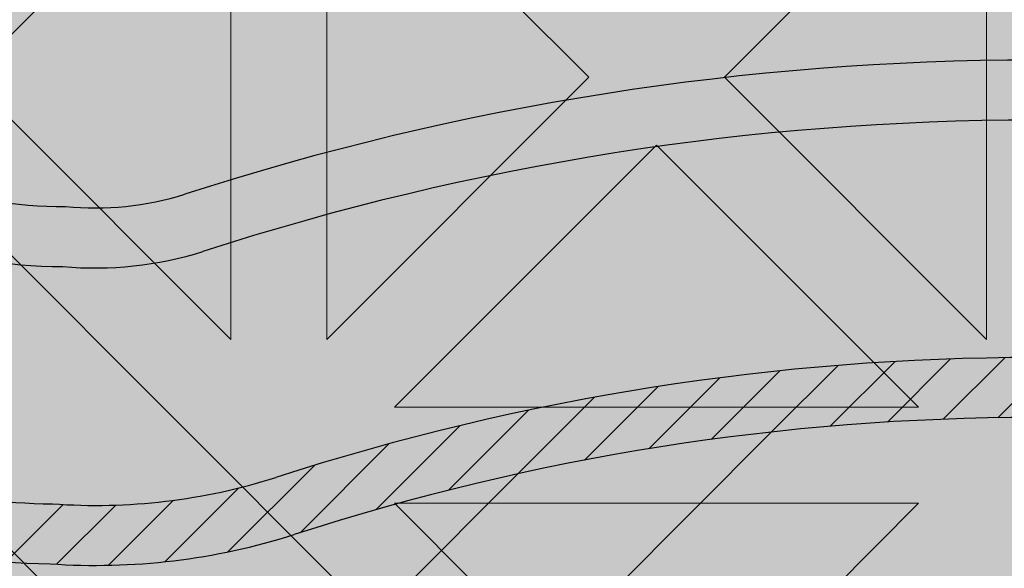
# Model space of a CAD drawing. Units: inches. Extents: x 844 to 2234, y 346 to 1084.
# Tile 20 of 93: x 1120.159 to 1122.777, y 703.603 to 705.06. Entities that reach past the tile are written whole.
import ezdxf

# ---------------------------------------------------------------- set-up
doc = ezdxf.new("R2010")
doc.units = ezdxf.units.IN
doc.header["$MEASUREMENT"] = 0
for name, color, linetype, lineweight in [('A-ANNO-DIMS', 2, 'Continuous', 18), ('furniture', 8, 'Continuous', 18), ('RA-AP-01$0$INT', 35, 'Continuous', 5)]:
    doc.layers.add(name, color=color, linetype=linetype, lineweight=lineweight)
doc.layers.add('RA-AP-01$0$FURN', color=3, linetype='Continuous')
doc.layers.add('RA-AP-01$0$WOOD', color=64, linetype='Continuous')
doc.styles.get("Standard").update_dxf_attribs({"font": 'arial.ttf'})
doc.dimstyles.get("Standard").update_dxf_attribs({"dimtxt": 6, "dimasz": 3, "dimexe": 0.18, "dimexo": 0.0625, "dimgap": 0.09, "dimtad": 0, "dimtih": 1, "dimtoh": 1, "dimdec": 1, "dimzin": 0, "dimdsep": 46, "dimlunit": 3, "dimtxsty": 'Standard', "dimblk": 'ARCHTICK', "dimcen": 0.09, "dimadec": 0, "dimazin": 0, "dimtfac": 1, "dimtdec": 1, "dimtofl": 0, "dimtmove": 0, "dimatfit": 3, "dimfxl": 1, "dimtolj": 1, "dimtzin": 0, "dimarcsym": 0})

# ---------------------------------------------------------------- blocks, each defined once
blk = doc.blocks.new('A$C18D01794')
at = {"layer": 'RA-AP-01$0$INT'}
h = blk.add_hatch(color=256, dxfattribs=at)
h.paths.add_polyline_path([(4.585917135068448, -7.856712009587804), (4.614201406330596, -7.856712009587056), (4.668846067270487, -7.802067348644738), (4.723490728212344, -7.856712009584164), (4.771774999457151, -7.856712009582887), (4.826419660396886, -7.80206734864072), (4.862780050090322, -7.838427738332541), (4.844495778842715, -7.856712009580965), (4.862780050090411, -7.856712009580482), (4.905206456960182, -7.814285602707865), (4.947632863832445, -7.856712009578238), (4.965917135079675, -7.856712009577755), (4.947632863831759, -7.838427738330656), (4.983993253523576, -7.802067348637219), (5.038637914464627, -7.856712009575829), (5.08692218571208, -7.856712009574554), (5.141566846649976, -7.802067348634224), (5.196211507589851, -7.856712009571666), (5.224495778822615, -7.856712009570916), (4.905206456953975, -7.537422687702283)])
h.paths.add_polyline_path([(4.895206456956031, -7.575706958950402), (4.895206456958921, -7.684996280828174), (4.840561796018589, -7.630351619890275)], flags=16)
h.paths.add_polyline_path([(4.915206456955638, -7.575706958949956), (4.969851117895509, -7.630351619887399), (4.915206456957609, -7.684996280827732)], flags=16)
h.paths.add_polyline_path([(4.826419660395175, -7.644493755514321), (4.881064321335613, -7.699138416452331), (4.771774999456703, -7.69913841645522)], flags=16)
h.paths.add_polyline_path([(4.983993253519558, -7.644493755510815), (5.038637914460456, -7.699138416449285), (4.929348592581548, -7.69913841645126)], flags=16)
h.paths.add_polyline_path([(4.881064321336025, -7.719138416452334), (4.826419660397532, -7.773783077393256), (4.771774999457062, -7.719138416455217)], flags=16)
h.paths.add_polyline_path([(4.929348592582019, -7.71913841645126), (5.038637914460982, -7.719138416449284), (4.983993253522945, -7.773783077389749)], flags=16)
h.paths.add_polyline_path([(4.895206456960191, -7.733280552075633), (4.895206456962115, -7.806001331460164), (4.876922185715016, -7.824285602708492), (4.840561796021581, -7.787925213016675)], flags=16)
h.paths.add_polyline_path([(4.915206456958487, -7.733280552075187), (4.969851117899527, -7.787925213013798), (4.933490728206909, -7.824285602708034), (4.9152064569598, -7.806001331461736)], flags=16)
h.paths.add_polyline_path([(4.757632863832376, -7.733280552079264), (4.812277524772842, -7.787925213017304), (4.757632863834348, -7.842569873958233)], flags=16)
h.paths.add_polyline_path([(4.737632863832376, -7.73328055207979), (4.737632863834348, -7.842569873958701), (4.682988202893906, -7.787925213020692)], flags=16)
h.paths.add_polyline_path([(5.05278005008503, -7.733280552072701), (5.052780050087917, -7.842569873951664), (4.998135389146995, -7.787925213013169)], flags=16)
h.paths.add_polyline_path([(5.072780050085024, -7.733280552072333), (5.127424711025931, -7.787925213010806), (5.072780050087916, -7.842569873951244)], flags=16)
h.paths.add_polyline_path([(4.935917135072783, -7.506712009583784), (5.255206456948811, -7.826001331459767), (5.255206456948932, -7.797717060211899), (5.200561796010279, -7.743072399273238), (5.255206456949403, -7.688427738334128), (5.25520645694961, -7.640143467086677), (5.200561796009787, -7.585498806146837), (5.236922185702417, -7.549138416454212), (5.255206456949919, -7.56742268770172), (5.255206456949998, -7.549138416454178), (5.212780050078687, -7.506712009583814), (5.25520645695036, -7.464285602712145), (5.255206456950438, -7.446001331464763), (5.236922185702424, -7.464285602712779), (5.200561796009796, -7.427925213020149), (5.255206456950753, -7.373280552079203), (5.25520645695096, -7.324996280834394), (5.200561796010322, -7.270351619893748), (5.255206456951428, -7.215706958952649), (5.255206456951547, -7.187422687705071)])
h.paths.add_polyline_path([(5.042988202883395, -7.42792521302065), (5.097632863823085, -7.373280552080975), (5.097632863822622, -7.482569873959883)], flags=16)
h.paths.add_polyline_path([(5.028846067259663, -7.442067348644384), (5.083490728198774, -7.496712009583504), (4.974201406321001, -7.496712009583035)], flags=16)
h.paths.add_polyline_path([(5.117632863823087, -7.37328055208089), (5.172277524762331, -7.42792521302015), (5.11763286382262, -7.482569873959851)], flags=16)
h.paths.add_polyline_path([(5.08349072819877, -7.516712009582191), (5.028846067259652, -7.571356670521302), (4.974201406320998, -7.516712009582638)], flags=16)
h.paths.add_polyline_path([(5.131774999446817, -7.35913841645716), (5.186419660386065, -7.413783077396415), (5.241064321325782, -7.359138416456712)], flags=17)
h.paths.add_polyline_path([(5.131774999446228, -7.496712009583703), (5.186419660386065, -7.442067348643883), (5.222780050079488, -7.478427738337313), (5.204495778832781, -7.496712009584014)], flags=16)
h.paths.add_polyline_path([(5.097632863822613, -7.530854145205813), (5.097632863823061, -7.640143467084723), (5.042988202883383, -7.585498806145032)], flags=16)
h.paths.add_polyline_path([(5.131774999446899, -7.339138416457162), (5.241064321325809, -7.339138416456712), (5.186419660386591, -7.284493755517479)], flags=17)
h.paths.add_polyline_path([(5.131774999446226, -7.516712009581999), (5.204495778830767, -7.516712009581702), (5.22278005007868, -7.534996280829206), (5.186419660386049, -7.571356670521828)], flags=16)
h.paths.add_polyline_path([(5.11763286382262, -7.530854145205852), (5.17227752476232, -7.585498806145562), (5.117632863823064, -7.64014346708481)], flags=16)
h.paths.add_polyline_path([(5.186419660386069, -7.599640941770585), (5.241064321325754, -7.654285602710281), (5.131774999446791, -7.654285602709814)], flags=16)
h.paths.add_polyline_path([(5.131774999446872, -7.674285602709813), (5.24106432132578, -7.674285602710282), (5.186419660386554, -7.728930263649504)], flags=16)
h.paths.add_polyline_path([(5.255206456951811, -7.126001331467467), (5.255206456951895, -7.106712009588038), (4.555206456956052, -7.106712009588038), (4.555206456956136, -7.12600133146746), (4.905206456953973, -7.476001331465289)])
h.paths.add_polyline_path([(4.983993253513404, -7.368930263651977), (4.92934859257295, -7.314285602713969), (5.03863791445186, -7.314285602711063)], flags=16)
h.paths.add_polyline_path([(4.969851117889988, -7.383072399276016), (4.915206456952556, -7.437717060215906), (4.915206456949648, -7.328427738338133)], flags=16)
h.paths.add_polyline_path([(4.929348592572535, -7.294285602713971), (4.983993253511019, -7.239640941773039), (5.038637914451496, -7.294285602711065)], flags=16)
h.paths.add_polyline_path([(5.052780050074912, -7.280143467087016), (4.998135389134438, -7.225498806148989), (5.052780050072919, -7.170854145208052)], flags=16)
h.paths.add_polyline_path([(5.07278005007491, -7.280143467086489), (5.072780050072918, -7.170854145207579), (5.127424711013374, -7.225498806145578)], flags=16)
h.paths.add_polyline_path([(4.89520645695295, -7.437717060216355), (4.840561796013067, -7.383072399278919), (4.895206456950961, -7.328427738338582)], flags=16)
h.paths.add_polyline_path([(4.915206456948365, -7.280143467090674), (4.915206456946434, -7.207422687704125), (4.933490728192729, -7.18913841645701), (4.969851117886972, -7.225498806149623)], flags=16)
h.paths.add_polyline_path([(4.881064321327021, -7.314285602715054), (4.82641966038902, -7.368930263655506), (4.771774999448108, -7.314285602717047)], flags=16)
h.paths.add_polyline_path([(4.895206456950073, -7.280143467091125), (4.840561796009022, -7.225498806152518), (4.876922185700835, -7.18913841645908), (4.895206456948749, -7.207422687706589)], flags=16)
h.paths.add_polyline_path([(4.983993253510392, -7.211356670525576), (4.947632863816944, -7.174996280833758), (4.965917135064043, -7.156712009585847), (5.038637914448995, -7.156712009584522)], flags=16)
h.paths.add_polyline_path([(4.881064321326543, -7.294285602715056), (4.771774999447578, -7.294285602717046), (4.826419660385607, -7.239640941776569)], flags=16)
h.paths.add_polyline_path([(4.905206456946447, -7.19913841645844), (4.862780050074785, -7.156712009587725), (4.947632863816685, -7.156712009586302)], flags=16)
h.paths.add_polyline_path([(5.14156684663679, -7.211356670521528), (5.086922185696452, -7.156712009583639), (5.196211507574223, -7.156712009581651)], flags=16)
h.paths.add_polyline_path([(4.8264196603837, -7.211356670529104), (4.771774999442643, -7.156712009590501), (4.8444957788276, -7.156712009588568), (4.862780050075511, -7.17499628083566)], flags=16)
h.paths.add_polyline_path([(4.812277524760289, -7.225498806153156), (4.757632863822258, -7.28014346709363), (4.757632863819352, -7.170854145214669)], flags=16)
h.paths.add_polyline_path([(4.73763286382226, -7.280143467093997), (4.682988202881349, -7.22549880615554), (4.737632863819352, -7.170854145215086)], flags=16)
h.paths.add_polyline_path([(4.723490728195188, -7.156712009591787), (4.668846067257299, -7.211356670532127), (4.614201406317417, -7.156712009594693)], flags=16)
h.paths.add_polyline_path([(4.597632863829262, -7.506712009583814), (4.555206456957951, -7.54913841645418), (4.555206456958029, -7.56742268770172), (4.573490728205535, -7.549138416454212), (4.609851117898167, -7.585498806146839), (4.555206456958338, -7.640143467086675), (4.555206456958546, -7.688427738334125), (4.60985111789767, -7.743072399273238), (4.555206456959015, -7.797717060211899), (4.555206456959138, -7.826001331459767), (4.874495778835167, -7.506712009583786), (4.5552064569564, -7.187422687705062), (4.555206456956523, -7.215706958952644), (4.609851117897629, -7.270351619893746), (4.555206456956988, -7.324996280834396), (4.555206456957198, -7.373280552079195), (4.609851117898153, -7.427925213020147), (4.573490728205528, -7.464285602712779), (4.555206456957507, -7.446001331464756), (4.555206456957585, -7.464285602712143)])
h.paths.add_polyline_path([(4.712780050085332, -7.482569873959882), (4.712780050084863, -7.373280552080972), (4.767424711024555, -7.42792521302065)], flags=16)
h.paths.add_polyline_path([(4.726922185709173, -7.496712009583504), (4.781566846648288, -7.442067348644384), (4.836211507586949, -7.496712009583033)], flags=16)
h.paths.add_polyline_path([(4.692780050085327, -7.482569873959851), (4.638135389145619, -7.427925213020149), (4.692780050084865, -7.373280552080892)], flags=16)
h.paths.add_polyline_path([(4.726922185709182, -7.516712009582191), (4.836211507586949, -7.51671200958264), (4.7815668466483, -7.571356670521304)], flags=16)
h.paths.add_polyline_path([(4.678637914461726, -7.496712009583706), (4.605917135075169, -7.496712009584014), (4.587632863828464, -7.478427738337311), (4.623993253521887, -7.442067348643881)], flags=16)
h.paths.add_polyline_path([(4.712780050085336, -7.530854145205816), (4.767424711024568, -7.585498806145034), (4.71278005008489, -7.640143467084724)], flags=16)
h.paths.add_polyline_path([(4.678637914461726, -7.516712009582001), (4.623993253521899, -7.571356670521829), (4.587632863829271, -7.534996280829206), (4.605917135077185, -7.5167120095817)], flags=16)
h.paths.add_polyline_path([(4.692780050085336, -7.530854145205848), (4.692780050084889, -7.64014346708481), (4.638135389145632, -7.585498806145562)], flags=16)
h.paths.add_polyline_path([(4.623993253521885, -7.413783077396415), (4.678637914461131, -7.359138416457161), (4.56934859258217, -7.359138416456712)], flags=17)
h.paths.add_polyline_path([(4.623993253521901, -7.599640941770568), (4.678637914461158, -7.654285602709814), (4.569348592582195, -7.654285602710281)], flags=16)
h.paths.add_polyline_path([(4.678637914461051, -7.339138416457162), (4.623993253521361, -7.284493755517479), (4.569348592582143, -7.339138416456712)], flags=17)
h.paths.add_polyline_path([(4.678637914461076, -7.674285602709813), (4.623993253521399, -7.728930263649504), (4.569348592582167, -7.674285602710281)], flags=16)
h = blk.add_hatch(color=256, dxfattribs=at)
h.paths.add_polyline_path([(4.905206456954232, -7.537422687702028), (4.874495778835232, -7.506712009583718), (4.555206456959138, -7.826001331459766), (4.555206456959269, -7.856712009588616), (4.585917135068449, -7.856712009587804)])
h.paths.add_polyline_path([(4.935917135072152, -7.506712009583152), (4.905206456953497, -7.537422687701806), (5.224495778822614, -7.856712009570917), (5.255206456948681, -7.856712009570104), (5.255206456948813, -7.826001331459768)])
h.paths.add_polyline_path([(5.255206456951549, -7.18742268770507), (5.255206456951813, -7.126001331467461), (4.905206456953563, -7.476001331465701), (4.935917135072559, -7.506712009584006)])
h.paths.add_polyline_path([(4.874495778835167, -7.506712009583785), (4.905206456953818, -7.476001331465132), (4.555206456956135, -7.126001331467458), (4.555206456956399, -7.187422687705064)])
h = blk.add_hatch(color=256, dxfattribs=at)
h.paths.add_polyline_path([(4.969851117891331, -7.630351619889621), (4.915206456952669, -7.575706958950966), (4.915206456952222, -7.684996280828739)])
h.paths.add_polyline_path([(4.895206456953064, -7.575706958950968), (4.840561796014413, -7.630351619889628), (4.895206456953533, -7.684996280828741)])
h.paths.add_polyline_path([(4.826419660390684, -7.644493755513362), (4.771774999451003, -7.699138416453052), (4.881064321329913, -7.699138416452587)])
h.paths.add_polyline_path([(4.881064321329884, -7.719138416452585), (4.771774999450921, -7.719138416453052), (4.82641966039018, -7.773783077392298)])
h.paths.add_polyline_path([(4.895206456953734, -7.733280552076196), (4.840561796013912, -7.787925213016031), (4.876922185707337, -7.824285602709455), (4.895206456954043, -7.806001331462747)])
h.paths.add_polyline_path([(4.862780050082808, -7.838427738332388), (4.826419660390178, -7.802067348639763), (4.771774999450351, -7.856712009579595), (4.844495778835303, -7.856712009579895)])
h.paths.add_polyline_path([(4.812277524766446, -7.787925213016036), (4.757632863827191, -7.733280552076788), (4.757632863826741, -7.842569873955747)])
h.paths.add_polyline_path([(4.737632863827191, -7.733280552076863), (4.682988202887508, -7.787925213016558), (4.737632863826743, -7.842569873955778)])
h.paths.add_polyline_path([(4.668846067263777, -7.802067348640287), (4.614201406325123, -7.856712009578949), (4.723490728202894, -7.856712009579402)])
h.paths.add_polyline_path([(4.905206456953846, -7.814285602708654), (4.862780050082654, -7.856712009579847), (4.947632863824561, -7.85671200958032)])
h.paths.add_polyline_path([(4.915206456952028, -7.733280552076195), (4.91520645695173, -7.806001331460731), (4.933490728199234, -7.824285602708648), (4.96985111789186, -7.787925213016022)])
h.paths.add_polyline_path([(5.038637914454841, -7.719138416453029), (4.929348592575874, -7.71913841645258), (4.983993253515593, -7.773783077392289)])
h.paths.add_polyline_path([(4.983993253515065, -7.644493755513352), (4.929348592575849, -7.699138416452582), (5.038637914454755, -7.699138416453031)])
h.paths.add_polyline_path([(5.052780050079843, -7.73328055207676), (4.998135389140595, -7.787925213016018), (5.052780050080309, -7.842569873955721)])
h.paths.add_polyline_path([(4.983993253516868, -7.802067348639752), (4.947632863824241, -7.838427738332383), (4.965917135071747, -7.856712009579888), (5.038637914456701, -7.856712009579572)])
h.paths.add_polyline_path([(5.127424711019533, -7.787925213016519), (5.072780050079843, -7.733280552076838), (5.07278005008031, -7.842569873955751)])
h.paths.add_polyline_path([(5.141566846643269, -7.802067348640248), (5.086922185704154, -7.85671200957937), (5.196211507581929, -7.856712009578901)])
for p, q in [((4.874495778835167, -7.506712009583786), (4.555206456959136, -7.826001331459769)), ((4.905206456953975, -7.537422687702283), (4.585917135071132, -7.856712009585121)), ((4.826419660395171, -7.644493755514321), (4.771774999456703, -7.69913841645522)), ((4.881064321335613, -7.699138416452333), (4.826419660395173, -7.64449375551432)), ((4.771774999456703, -7.69913841645522), (4.881064321335613, -7.699138416452333)), ((4.771774999457064, -7.719138416455219), (4.881064321336027, -7.719138416452333)), ((4.771774999457064, -7.719138416455219), (4.826419660397532, -7.773783077393256)), ((4.881064321336027, -7.719138416452333), (4.826419660397532, -7.773783077393256)), ((4.682988202893908, -7.78792521302069), (4.737632863832376, -7.733280552079792)), ((4.737632863832376, -7.733280552079792), (4.737632863834348, -7.842569873958701)), ((4.757632863832376, -7.733280552079266), (4.812277524772842, -7.787925213017302)), ((4.757632863832376, -7.733280552079266), (4.757632863834348, -7.842569873958229)), ((4.895206456960191, -7.73328055207563), (4.840561796021581, -7.787925213016675)), ((4.895206456962113, -7.806001331460581), (4.895206456960191, -7.73328055207563)), ((4.737632863834348, -7.842569873958701), (4.682988202893906, -7.787925213020692)), ((4.757632863834348, -7.842569873958229), (4.812277524772842, -7.787925213017302)), ((4.840561796021581, -7.787925213016674), (4.876922185715016, -7.824285602708492))]:
    blk.add_line(p, q, dxfattribs=at)
blk = doc.blocks.new('A$C32926AE1')
at = {"layer": 'RA-AP-01$0$WOOD'}
h = blk.add_hatch(color=256, dxfattribs=at)
h.dxf.hatch_style = 1
h.paths.add_polyline_path([(5.157430609644524, 4.573483066760929, -0.1009492694046607), (5.155401577623758, 4.593365984175333, -0.1842662638101597), (5.172249623284174, 4.638795604568598, 0.2056608120311276), (5.179560981299304, 4.661316324430096, 0.3614336704623542), (5.134352340494423, 4.706524965234944, 0.2056608120311297), (5.111831620632933, 4.699213607219793, -0.1842662638101113), (5.066402000239693, 4.682365561559342, -0.1055311479399994), (5.045656153913092, 4.68467289944697, 0.1567636581983829), (4.763886414745334, 4.684672899446966, -0.1055311479399895), (4.743140568418733, 4.68236556155934, -0.1842662638100833), (4.6977109480255, 4.69921360721979, 0.2056608120302612), (4.675190228164109, 4.706524965234949, 0.3614336704708441), (4.629981587358889, 4.66131632442871, 0.2056608120245944), (4.637292945374126, 4.638795604567974, -0.1842662638101024), (4.654140991034615, 4.59336598417475, -0.1009492694055169), (4.652111959013835, 4.573483066760181, 0.021410119221476), (4.629748025606143, 4.156712009541676, 0.0214101192214795), (4.652111959013809, 3.739940952323101, -0.1009492694059586), (4.654140991034615, 3.720058034908448, -0.1842662638100975), (4.637292945374126, 3.674628414515226, 0.2056608120245705), (4.629981587358889, 3.652107694654492, 0.3614336704708879), (4.675190228164113, 3.606899053848249, 0.2056608120302384), (4.697710948025501, 3.614210411863408, -0.1842662638100995), (4.743140568418738, 3.63105845752386, -0.1055311479402541), (4.763886414745388, 3.628751119636215, 0.1567636581983776), (5.045656153913137, 3.628751119636244, -0.1055311479397538), (5.066402000239692, 3.631058457523857, -0.1842662638101067), (5.111831620632931, 3.614210411863407, 0.2056608120310924), (5.134352340494417, 3.606899053848256, 0.3614336704624001), (5.179560981299307, 3.652107694653103, 0.2056608120311314), (5.172249623284175, 3.6746284145146, -0.1842662638101402), (5.155401577623758, 3.72005803490786, -0.1009492694051366), (5.15743060964455, 3.739940952322354, 0.0214101192215073), (5.179794543052287, 4.156712009541468, 0.0214101192215252)])
h.paths.add_polyline_path([(4.639748609479751, 4.156712009541513, 0.0213537860821624), (4.661970494867118, 3.741887061152232, -0.094075836301374), (4.664143710413708, 3.7196126951003, -0.1824818158568985), (4.644813765429836, 3.668037719127816, 0.2056608120245319), (4.639939526753007, 3.653023905887301, 0.3614336704710246), (4.676106439397173, 3.616856993242342, 0.2056608120302234), (4.691120252638095, 3.621731231919122, -0.1824818158602558), (4.742695228611606, 3.641061176902986, -0.1029891339458722), (4.766991894714349, 3.638256818950944, 0.156709409989566), (5.042550673941472, 3.638256818950105, -0.102989133958497), (5.066847340047078, 3.641061176902949, -0.1824818158594995), (5.118422316020358, 3.621731231919103, 0.2056608120311416), (5.133436129261316, 3.616856993242346, 0.3614336704621468), (5.169603041905217, 3.653023905886178, 0.2056608120310986), (5.164728803228477, 3.668037719127177, -0.1824818158565612), (5.145398858244737, 3.719612695099578, -0.0940758363009313), (5.147572073791232, 3.741887061151398, 0.0213537860822023), (5.169793959178681, 4.156712009541451, 0.0213537860822226), (5.147572073791203, 4.571536957931898, -0.0940758363005034), (5.145398858244737, 4.59381132398362, -0.1824818158565587), (5.164728803228476, 4.645386299956021, 0.2056608120311045), (5.169603041905216, 4.66040011319702, 0.3614336704621845), (5.133436129261313, 4.696567025840856, 0.2056608120310773), (5.118422316020359, 4.691692787164098, -0.182481815859508), (5.066847340047078, 4.67236284218025, -0.1029891339584606), (5.04255067394148, 4.675167200133092, 0.156709409989566), (4.766991894714357, 4.675167200132257, -0.1029891339458842), (4.742695228611611, 4.672362842180213, -0.1824818158602725), (4.691120252638095, 4.691692787164077, 0.2056608120302152), (4.676106439397174, 4.696567025840858, 0.3614336704710363), (4.639939526753005, 4.660400113195899, 0.2056608120245495), (4.644813765429837, 4.645386299955384, -0.1824818158568934), (4.664143710413708, 4.593811323982902, -0.0940758363009187), (4.661970494867149, 4.571536957931074, 0.021353786082177)], flags=16)
h.paths.add_polyline_path([(5.129794543052235, 4.432167055276933, -0.0141661062790638), (5.130152669293814, 4.156927903047693, -0.0141661062790647), (5.129794543052234, 3.881688750818433, -0.0785247771143638), (5.10979738006795, 3.755143611847103, 0.0945969212073497), (5.105408519571111, 3.717898134952927, 0.1043170707844957), (5.116074640131521, 3.670385395016088, 0.1043170707864965), (5.068561900193738, 3.681051515576561, 0.09459692119553), (5.031316423304057, 3.676662655080835, -0.1580239521427272), (4.778226145355827, 3.676662655080367, 0.0945969211986668), (4.740980668464973, 3.681051515576592, 0.1043170707882822), (4.693467928526415, 3.670385395015844, 0.1043170707867916), (4.704134049087309, 3.717898134953662, 0.0945969211972894), (4.69974518859162, 3.755143611844042, -0.0785247771163196), (4.679748025606343, 3.881688750818406, -0.0141661062790663), (4.679389899364763, 4.156927903047693, -0.0141661062790672), (4.679748025606343, 4.432167055276998, -0.0785247771163064), (4.699745188591625, 4.55871219425134, 0.094596921197333), (4.704134049087308, 4.595957671141738, 0.1043170707867205), (4.693467928526416, 4.643470411079523, 0.1043170707882628), (4.740980668464965, 4.632804290518776, 0.0945969211988114), (4.778226145355874, 4.637193151015016, -0.158023952142669), (5.031316423304015, 4.637193151014546, 0.0945969211956361), (5.068561900193736, 4.632804290518806, 0.1043170707864979), (5.11607464013152, 4.643470411079278, 0.1043170707844617), (5.105408519571112, 4.595957671142455, 0.0945969212074597), (5.109797380067959, 4.558712194248236, -0.0785247771143467)], flags=0)
h.paths.add_polyline_path([(5.119794532311105, 4.432259799204851, -0.0142000800617244), (5.120156169157484, 4.156927903047701, -0.0142000800617277), (5.119794532311105, 3.881596006890482, -0.0784894509520253), (5.100273383573699, 3.758192358677797, 0.0940138827242913), (5.095413455884425, 3.717477693979438, 0.0606271852308753), (5.099615656341024, 3.686844378806616, 0.0606271852322524), (5.068982341167493, 3.691046579263239, 0.0940138827010453), (5.028267676478798, 3.686186651576848, -0.1580706864508061), (4.781274892180912, 3.686186651576435, 0.0940138827026903), (4.740560227491556, 3.691046579263279, 0.0606271852339895), (4.709926912317155, 3.686844378806508, 0.0606271852329405), (4.714129112773991, 3.717477693980356, 0.094013882701304), (4.709269185087677, 3.758192358669163, -0.0784894509577193), (4.689748036347473, 3.881596006890469, -0.014200080061729), (4.689386399501094, 4.156927903047709, -0.0142000800617217), (4.689748036347473, 4.432259799204808, -0.078489450957724), (4.709269185087651, 4.555663447426125, 0.0940138827014585), (4.714129112773992, 4.596378112114996, 0.0606271852329731), (4.709926912317154, 4.62701142728886, 0.0606271852340196), (4.74056022749157, 4.622809226832087, 0.0940138827024997), (4.781274892180847, 4.627669154518912, -0.1580706864508359), (5.028267676478777, 4.627669154518526, 0.0940138827010946), (5.068982341167492, 4.622809226832129, 0.060627185232254), (5.099615656341024, 4.627011427288751, 0.0606271852308727), (5.095413455884425, 4.59637811211593, 0.0940138827241088), (5.100273383573675, 4.555663447417647, -0.0784894509520978)], flags=0)
h.paths.add_polyline_path([(5.06978912287499, 4.430218106756144, -0.014241683694547), (5.070173729147532, 4.156927903047672, -0.0142416836945458), (5.06978912287499, 3.883637699339223, -0.0800609523125196), (5.052662118612511, 3.773463122773442, 0.0526421978001116), (5.04590916754064, 3.740550867606997, 0.0526421977992423), (5.012996912374707, 3.73379791653534, -0.1583028414718258), (4.796545656286308, 3.73379791653451, 0.0526421978034211), (4.763633401117837, 3.740550867607021, 0.0526421978018622), (4.756880450045755, 3.773463122774558, -0.0800609523117106), (4.739753445783639, 3.883637699339268, -0.0142416836945435), (4.739368839511098, 4.156927903047671, -0.0142416836945477), (4.739753445783639, 4.430218106756155, -0.0800609523116345), (4.75688045004574, 4.540392683320762, 0.052642197801941), (4.763633401117837, 4.573304938488346, 0.0526421978035071), (4.796545656286361, 4.580057889560873, -0.1583028414717561), (5.012996912374669, 4.580057889560039, 0.0526421977993048), (5.04590916754064, 4.57330493848837, 0.0526421978002057), (5.052662118612529, 4.540392683321868, -0.080060952312477)], flags=0)
h.paths.add_polyline_path([(5.049789715110557, 4.43038092723357, -0.0143097550741839), (5.05018085590259, 4.156927903047715, -0.0143097550741854), (5.049789715110558, 3.883474878861827, -0.0800685599149176), (5.03362098255317, 3.779581877367999, 0.0306258898956367), (5.028241146483733, 3.758218888663947, 0.0306258898977031), (5.006878157778253, 3.75283905259408, -0.1583983521624096), (4.802664410878162, 3.752839052594731, 0.0306258898946014), (4.781301422174808, 3.758218888663924, 0.0306258898967912), (4.775921586105202, 3.779581877368794, -0.080068559914251), (4.759752853548071, 3.883474878861786, -0.0143097550741854), (4.759361712756037, 4.156927903047671, -0.0143097550741854), (4.759752853548071, 4.430380927233557, -0.0800685599142479), (4.775921586105193, 4.534273928726546, 0.0306258898968306), (4.781301422174808, 4.555636917431444, 0.0306258898945754), (4.802664410878143, 4.561016753500631, -0.1583983521624168), (5.006878157778244, 4.561016753501291, 0.0306258898977177), (5.028241146483733, 4.555636917431421, 0.0306258898958182), (5.03362098255321, 4.534273928727244, -0.080068559914796)], flags=0)
h.paths.add_polyline_path([(4.999766070382627, 4.428171244713864, -0.0143443147609634), (5.000198441819402, 4.156927903047689, -0.0143443147609612), (4.999766070382627, 3.885684561381556, -0.0784641635803329), (4.987356730658798, 3.799103304488872, -0.1506053783831347), (4.822185837999821, 3.79910330448882, -0.0784641635803318), (4.809776498276007, 3.885684561381509, -0.014344314760963), (4.809344126839227, 4.156927903047677, -0.0143443147609645), (4.809776498276007, 4.428171244713873, -0.0784641635803192), (4.822185837999822, 4.514752501606549, -0.1506053783831338), (4.987356730658798, 4.514752501606494, -0.078464163580285)], flags=0)
h.paths.add_polyline_path([(4.979755254238824, 4.42764379880488, -0.0143772539198268), (4.980205517789977, 4.156927903047693, -0.0143772539198275), (4.979755254238824, 3.886212007290489, -0.0689242507424422), (4.971183264704897, 3.815276770442801, -0.1296645318904179), (4.838359303953726, 3.815276770442746, -0.0689242507424186), (4.829787314419809, 3.886212007290419, -0.0143772539198292), (4.829337050868653, 4.156927903047653, -0.0143772539198325), (4.829787314419809, 4.427643798804946, -0.0689242507424211), (4.838359303953725, 4.498579035652621, -0.1296645318904187), (4.971183264704897, 4.498579035652565, -0.0689242507424401)], flags=0)
h = blk.add_hatch(color=256, dxfattribs=at)
h.dxf.hatch_style = 1
h.paths.add_polyline_path([(5.145398858244737, 4.59381132398362, -0.1824818158565616), (5.164728803228476, 4.645386299956021, 0.2056608120311045), (5.169603041905216, 4.66040011319702, 0.3614336704621845), (5.133436129261313, 4.696567025840856, 0.2056608120310773), (5.118422316020359, 4.691692787164098, -0.182481815859508), (5.066847340047078, 4.67236284218025, -0.1029891339584606), (5.04255067394148, 4.675167200133092, 0.156709409989566), (4.766991894714357, 4.675167200132257, -0.1029891339458842), (4.742695228611611, 4.672362842180213, -0.1824818158602725), (4.691120252638095, 4.691692787164077, 0.2056608120302152), (4.676106439397174, 4.696567025840858, 0.3614336704710363), (4.639939526753005, 4.660400113195899, 0.2056608120245495), (4.644813765429837, 4.645386299955384, -0.1824818158568934), (4.664143710413708, 4.593811323982902, -0.0940758363009187), (4.661970494867149, 4.571536957931074, 0.0213537860821772), (4.639748609479751, 4.156712009541507, 0.0213537860821625), (4.661970494867119, 3.741887061152226, -0.0940758363013071), (4.664143710413708, 3.719612695100309, -0.1824818158569294), (4.644813765429836, 3.668037719127816, 0.2056608120245319), (4.639939526753007, 3.653023905887301, 0.3614336704710246), (4.676106439397173, 3.616856993242342, 0.2056608120302234), (4.691120252638095, 3.621731231919122, -0.1824818158602558), (4.742695228611606, 3.641061176902986, -0.1029891339458722), (4.766991894714349, 3.638256818950944, 0.156709409989566), (5.042550673941472, 3.638256818950105, -0.102989133958497), (5.066847340047078, 3.641061176902949, -0.1824818158594995), (5.118422316020358, 3.621731231919103, 0.2056608120311416), (5.133436129261316, 3.616856993242346, 0.3614336704621468), (5.169603041905217, 3.653023905886178, 0.2056608120310986), (5.164728803228477, 3.668037719127177, -0.1824818158565612), (5.145398858244737, 3.719612695099578, -0.0940758363009313), (5.147572073791232, 3.741887061151398, 0.0213537860822023), (5.169793959178681, 4.156712009541451, 0.0213537860822226), (5.147572073791203, 4.571536957931898, -0.0940758363004996)])
h.paths.add_polyline_path([(5.109797380067958, 4.55871219424824, -0.0785247771143472), (5.129794543052234, 4.432167055276936, -0.0141661062790644), (5.130152669293814, 4.156927903047685, -0.014166106279066), (5.129794543052234, 3.881688750818401, -0.0785247771143517), (5.109797380067946, 3.755143611847092, 0.0945969212073132), (5.105408519571111, 3.717898134952929, 0.1043170707844995), (5.116074640131521, 3.670385395016088, 0.1043170707864965), (5.068561900193738, 3.681051515576561, 0.09459692119553), (5.031316423304057, 3.676662655080835, -0.1580239521427272), (4.778226145355827, 3.676662655080367, 0.0945969211986668), (4.740980668464973, 3.681051515576592, 0.1043170707882822), (4.693467928526415, 3.670385395015844, 0.1043170707867916), (4.704134049087309, 3.717898134953662, 0.0945969211972894), (4.69974518859162, 3.755143611844042, -0.0785247771163196), (4.679748025606343, 3.881688750818406, -0.0141661062790663), (4.679389899364763, 4.156927903047693, -0.0141661062790672), (4.679748025606343, 4.432167055276998, -0.0785247771163064), (4.699745188591625, 4.55871219425134, 0.094596921197333), (4.704134049087308, 4.595957671141738, 0.1043170707867205), (4.693467928526416, 4.643470411079523, 0.1043170707882628), (4.740980668464965, 4.632804290518776, 0.0945969211988114), (4.778226145355874, 4.637193151015016, -0.158023952142669), (5.031316423304015, 4.637193151014546, 0.0945969211956361), (5.068561900193736, 4.632804290518806, 0.1043170707864979), (5.11607464013152, 4.643470411079278, 0.1043170707844617), (5.105408519571112, 4.595957671142455, 0.0945969212074504)], flags=16)
h.paths.add_polyline_path([(5.100273383573655, 4.55566344741771, -0.0784894509521388), (5.119794532311105, 4.432259799204852, -0.0142000800617252), (5.120156169157484, 4.156927903047686, -0.014200080061726), (5.119794532311105, 3.881596006890502, -0.0784894509520446), (5.100273383573696, 3.758192358677786, 0.0940138827242721), (5.095413455884425, 3.717477693979436, 0.0606271852308692), (5.099615656341024, 3.686844378806616, 0.0606271852322522), (5.068982341167493, 3.691046579263239, 0.0940138827010453), (5.028267676478798, 3.686186651576848, -0.1580706864508061), (4.781274892180912, 3.686186651576435, 0.0940138827026903), (4.740560227491556, 3.691046579263279, 0.0606271852339895), (4.709926912317155, 3.686844378806508, 0.0606271852329405), (4.714129112773991, 3.717477693980356, 0.094013882701304), (4.709269185087677, 3.758192358669163, -0.0784894509577193), (4.689748036347473, 3.881596006890469, -0.014200080061729), (4.689386399501094, 4.156927903047709, -0.0142000800617217), (4.689748036347473, 4.432259799204808, -0.078489450957724), (4.709269185087651, 4.555663447426125, 0.0940138827014585), (4.714129112773992, 4.596378112114996, 0.0606271852329731), (4.709926912317154, 4.62701142728886, 0.0606271852340196), (4.74056022749157, 4.622809226832087, 0.0940138827024997), (4.781274892180847, 4.627669154518912, -0.1580706864508359), (5.028267676478777, 4.627669154518526, 0.0940138827010946), (5.068982341167492, 4.622809226832129, 0.060627185232254), (5.099615656341024, 4.627011427288751, 0.0606271852308727), (5.095413455884425, 4.59637811211593, 0.094013882723957)], flags=0)
h.paths.add_polyline_path([(5.04590916754064, 4.57330493848837, 0.0526421978002057), (5.052662118612529, 4.540392683321868, -0.0800609523124783), (5.06978912287499, 4.430218106756142, -0.0142416836945469), (5.070173729147532, 4.156927903047672, -0.0142416836945458), (5.06978912287499, 3.883637699339223, -0.0800609523125196), (5.052662118612511, 3.773463122773442, 0.0526421978001116), (5.04590916754064, 3.740550867606997, 0.0526421977992423), (5.012996912374707, 3.73379791653534, -0.1583028414718258), (4.796545656286308, 3.73379791653451, 0.0526421978034211), (4.763633401117837, 3.740550867607021, 0.0526421978018622), (4.756880450045755, 3.773463122774558, -0.0800609523117106), (4.739753445783639, 3.883637699339268, -0.0142416836945435), (4.739368839511098, 4.156927903047671, -0.0142416836945477), (4.739753445783639, 4.430218106756155, -0.0800609523116345), (4.75688045004574, 4.540392683320762, 0.052642197801941), (4.763633401117837, 4.573304938488346, 0.0526421978035071), (4.796545656286361, 4.580057889560873, -0.1583028414717561), (5.012996912374669, 4.580057889560039, 0.0526421977993048)], flags=0)
h.paths.add_polyline_path([(5.028241146483733, 4.555636917431422, 0.0306258898956949), (5.033620982553182, 4.534273928727329, -0.0800685599148649), (5.049789715110557, 4.430380927233569, -0.0143097550741839), (5.05018085590259, 4.156927903047715, -0.0143097550741854), (5.049789715110558, 3.883474878861827, -0.0800685599149176), (5.03362098255317, 3.779581877367999, 0.0306258898956367), (5.028241146483733, 3.758218888663947, 0.0306258898977031), (5.006878157778253, 3.75283905259408, -0.1583983521624096), (4.802664410878162, 3.752839052594731, 0.0306258898946014), (4.781301422174808, 3.758218888663924, 0.0306258898967912), (4.775921586105202, 3.779581877368794, -0.080068559914251), (4.759752853548071, 3.883474878861786, -0.0143097550741854), (4.759361712756037, 4.156927903047671, -0.0143097550741854), (4.759752853548071, 4.430380927233557, -0.0800685599142479), (4.775921586105193, 4.534273928726546, 0.0306258898968306), (4.781301422174808, 4.555636917431444, 0.0306258898945754), (4.802664410878143, 4.561016753500631, -0.1583983521624168), (5.006878157778244, 4.561016753501291, 0.0306258898977174)], flags=0)
h.paths.add_polyline_path([(4.987356730658798, 4.514752501606494, -0.0784641635803018), (4.999766070382627, 4.428171244713845, -0.0143443147609637), (5.000198441819402, 4.156927903047665, -0.0143443147609622), (4.999766070382628, 3.885684561381514, -0.0784641635802952), (4.987356730658797, 3.799103304488872, -0.1506053783831338), (4.822185837999821, 3.799103304488819, -0.0784641635803342), (4.809776498276007, 3.885684561381512, -0.0143443147609628), (4.809344126839227, 4.156927903047676, -0.0143443147609646), (4.809776498276007, 4.428171244713873, -0.0784641635803192), (4.822185837999822, 4.514752501606549, -0.1506053783831338)], flags=0)
h.paths.add_polyline_path([(4.971183264704897, 4.498579035652566, -0.0689242507424384), (4.979755254238824, 4.427643798804883, -0.0143772539198276), (4.980205517789977, 4.15692790304768, -0.0143772539198258), (4.979755254238823, 3.88621200729051, -0.0689242507424628), (4.971183264704897, 3.815276770442801, -0.129664531890417), (4.838359303953726, 3.815276770442746, -0.0689242507424186), (4.829787314419809, 3.886212007290419, -0.0143772539198292), (4.829337050868653, 4.156927903047653, -0.0143772539198325), (4.829787314419809, 4.427643798804946, -0.0689242507424211), (4.838359303953725, 4.498579035652621, -0.1296645318904187)], flags=0)
h = blk.add_hatch(dxfattribs=at)
h.set_pattern_fill('ANSI31', color=256, scale=0.05, style=0)
h.set_pattern_definition([(45, (0, 0), (-0.0044194173824159, 0.0044194173824159), [])])
h.paths.add_polyline_path([(5.130152669293814, 4.156927903047704, 0.0141661062790657), (5.129794543052234, 4.432167055276982, 0.0777827904001433), (5.110168979996553, 4.557559993161921, -0.0976515123401879), (5.105408519571111, 4.595957671142454, -0.1043170707844687), (5.116074640131522, 4.64347041107928), (5.099615656341024, 4.627011427288751, 0.0606271852308727), (5.095413455884425, 4.59637811211593, 0.0940138827241088), (5.100273383573675, 4.555663447417647, -0.0784894509520972), (5.119794532311105, 4.432259799204852, -0.0142000800617252), (5.120156169157484, 4.156927903047686, -0.014200080061726), (5.119794532311105, 3.881596006890502, -0.0784894509520446), (5.100273383573696, 3.758192358677786, 0.0940138827242721), (5.095413455884425, 3.717477693979436, 0.0606271852308692), (5.099615656341024, 3.686844378806616), (5.116074640131519, 3.67038539501609, -0.1043170707844594), (5.105408519571112, 3.717898134952912, -0.0976515123401594), (5.11016897999655, 3.756295812933435, 0.0777827904001654), (5.129794543052234, 3.881688750818409, 0.0141661062790665)])
h.paths.add_polyline_path([(5.030164222210597, 3.676291055149937, -0.0976515123472002), (5.068561900193739, 3.681051515576561, -0.1043170707864927), (5.116074640131521, 3.670385395016088), (5.099615656341024, 3.686844378806616, 0.0606271852322522), (5.068982341167493, 3.691046579263239, 0.0940138827010453), (5.028267676478798, 3.686186651576848, -0.1580706864508061), (4.781274892180912, 3.686186651576435, 0.0940138827026903), (4.740560227491556, 3.691046579263279, 0.0606271852339913), (4.709926912317154, 3.686844378806508), (4.693467928526416, 3.670385395015845, -0.1043170707882796), (4.740980668464973, 3.681051515576592, -0.0976515123427246), (4.779378346446416, 3.676291055150394, 0.156512506893803)])
h.paths.add_polyline_path([(4.689748036347473, 3.881596006890472, -0.014200080061729), (4.689386399501094, 4.156927903047712, -0.0142000800617195), (4.689748036347473, 4.432259799204768, -0.078489450957742), (4.709269185087648, 4.555663447426114, 0.0940138827014821), (4.714129112773992, 4.596378112114995, 0.0606271852329748), (4.709926912317154, 4.62701142728886), (4.693467928526414, 4.643470411079524, -0.1043170707867939), (4.704134049087309, 4.595957671141706, -0.09765151234893), (4.699373588660725, 4.557559993157876, 0.0777827903975372), (4.679748025606343, 4.432167055276987, 0.0141661062790675), (4.679389899364763, 4.156927903047675, 0.0141661062790641), (4.679748025606343, 3.88168875081843, 0.0777827903975637), (4.699373588660724, 3.756295812937497, -0.0976515123490278), (4.704134049087308, 3.717898134953629, -0.1043170707867196), (4.693467928526416, 3.670385395015845), (4.709926912317155, 3.686844378806508, 0.0606271852329413), (4.714129112773991, 3.717477693980357, 0.0940138827013084), (4.709269185087676, 3.758192358669166, -0.0784894509577192)])
h.paths.add_polyline_path([(4.779378346446434, 4.63756475094498, -0.0976515123427943), (4.740980668464964, 4.632804290518776, -0.1043170707882609), (4.693467928526416, 4.643470411079523), (4.709926912317154, 4.62701142728886, 0.0606271852340196), (4.74056022749157, 4.622809226832087, 0.0940138827024997), (4.781274892180847, 4.627669154518912, -0.1580706864508359), (5.028267676478777, 4.627669154518526, 0.0940138827010946), (5.068982341167492, 4.622809226832129, 0.060627185232254), (5.099615656341024, 4.627011427288751), (5.116074640131521, 4.643470411079279, -0.1043170707865022), (5.068561900193735, 4.632804290518806, -0.0976515123475899), (5.030164222210446, 4.637564750945479, 0.1565125068936924)])
h = blk.add_hatch(dxfattribs=at)
h.set_pattern_fill('ANSI32', color=256, scale=0.2, style=0)
h.set_pattern_definition([(45, (0, 0), (-0.0530330085889911, 0.0530330085889911), []), (45, (0.035355339, 0), (-0.0530330085889911, 0.0530330085889911), [])])
h.paths.add_polyline_path([(5.119794532311105, 4.432259799204823, 0.0777015974868765), (5.10065834347252, 4.554469821747928, -0.0968902511992216), (5.095413455884425, 4.596378112115931, -0.060627185230871), (5.099615656341024, 4.627011427288751, -0.060627185232254), (5.068982341167492, 4.622809226832129, -0.0968902512198245), (5.027074050790956, 4.628054114423209, 0.1564657949319105), (4.782468517866163, 4.628054114422785, -0.0968902512152247), (4.740560227491555, 4.622809226832088, -0.0606271852339878), (4.709926912317155, 4.627011427288859, -0.0606271852329413), (4.714129112773991, 4.596378112115011, -0.0968902512205338), (4.708884225182929, 4.554469821738175, 0.0777015974804443), (4.689748036347473, 4.43225979920482, 0.0142000800617215), (4.689386399501094, 4.156927903047726, 0.0142000800617273), (4.689748036347473, 3.88159600689052, 0.077701597480541), (4.708884225182985, 3.759385984357019, -0.096890251220082), (4.714129112773992, 3.717477693980371, -0.0606271852329731), (4.709926912317154, 3.686844378806507, -0.060627185233988), (4.740560227491554, 3.691046579263279, -0.0968902512152569), (4.782468517866175, 3.685801691672578, 0.1564657949319236), (5.027074050790988, 3.685801691672169, -0.0968902512197451), (5.068982341167491, 3.691046579263239, -0.0606271852322557), (5.099615656341024, 3.686844378806616, -0.0606271852308727), (5.095413455884425, 3.717477693979438, -0.0968902511991229), (5.100658343472507, 3.7593859843474, 0.0777015974868745), (5.119794532311105, 3.8815960068905, 0.014200080061726), (5.120156169157484, 4.156927903047685, 0.0142000800617238)])
h.paths.add_polyline_path([(5.070173729147531, 4.156927903047684, -0.0142416836945481), (5.06978912287499, 3.883637699339191, -0.0800609523125107), (5.052662118612505, 3.773463122773424, 0.0526421978000811), (5.04590916754064, 3.740550867606997, 0.0526421977993214), (5.012996912374658, 3.733797916535325, -0.1583028414717916), (4.796545656286304, 3.733797916534512, 0.0526421978034138), (4.763633401117837, 3.740550867607021, 0.0526421978018622), (4.756880450045755, 3.773463122774558, -0.0800609523117106), (4.739753445783639, 3.883637699339268, -0.0142416836945435), (4.739368839511098, 4.156927903047671, -0.0142416836945477), (4.739753445783639, 4.430218106756155, -0.0800609523116345), (4.75688045004574, 4.540392683320762, 0.052642197801941), (4.763633401117837, 4.573304938488346, 0.0526421978035071), (4.796545656286361, 4.580057889560873, -0.1583028414717561), (5.012996912374669, 4.580057889560039, 0.0526421977993048), (5.04590916754064, 4.57330493848837, 0.0526421978002057), (5.052662118612529, 4.540392683321868, -0.0800609523124783), (5.06978912287499, 4.430218106756142, -0.0142416836945463)], flags=16)
h.paths.add_polyline_path([(5.050180855902591, 4.156927903047686, -0.0143097550741856), (5.049789715110558, 3.883474878861795, -0.0800685599148126), (5.033620982553202, 3.7795818773681, 0.0306258898957837), (5.028241146483733, 3.758218888663947, 0.0306258898977031), (5.006878157778253, 3.75283905259408, -0.1583983521624096), (4.802664410878162, 3.752839052594731, 0.0306258898946014), (4.781301422174808, 3.758218888663924, 0.0306258898967912), (4.775921586105202, 3.779581877368794, -0.080068559914251), (4.759752853548071, 3.883474878861786, -0.0143097550741854), (4.759361712756037, 4.156927903047671, -0.0143097550741854), (4.759752853548071, 4.430380927233557, -0.0800685599142479), (4.775921586105193, 4.534273928726546, 0.0306258898968306), (4.781301422174808, 4.555636917431444, 0.0306258898945754), (4.802664410878143, 4.561016753500631, -0.1583983521624168), (5.006878157778244, 4.561016753501291, 0.0306258898977177), (5.028241146483733, 4.555636917431421, 0.0306258898958182), (5.03362098255321, 4.534273928727244, -0.0800685599147973), (5.049789715110557, 4.430380927233568, -0.0143097550741854)], flags=0)
h.paths.add_polyline_path([(5.000198441819402, 4.15692790304769, -0.0143443147609622), (4.999766070382627, 3.885684561381539, -0.0784641635803169), (4.987356730658798, 3.799103304488873, -0.1506053783831347), (4.822185837999821, 3.79910330448882, -0.0784641635803318), (4.809776498276007, 3.885684561381509, -0.014344314760963), (4.809344126839227, 4.156927903047677, -0.0143443147609645), (4.809776498276007, 4.428171244713873, -0.0784641635803192), (4.822185837999822, 4.514752501606549, -0.1506053783831338), (4.987356730658798, 4.514752501606494, -0.0784641635803018), (4.999766070382627, 4.428171244713845, -0.0143443147609624)], flags=0)
h.paths.add_polyline_path([(4.980205517789976, 4.156927903047707, -0.0143772539198295), (4.979755254238824, 3.886212007290466, -0.06892425074242), (4.971183264704897, 3.815276770442801, -0.129664531890417), (4.838359303953726, 3.815276770442746, -0.0689242507424186), (4.829787314419809, 3.886212007290419, -0.0143772539198292), (4.829337050868653, 4.156927903047653, -0.0143772539198325), (4.829787314419809, 4.427643798804946, -0.0689242507424211), (4.838359303953725, 4.498579035652621, -0.1296645318904187), (4.971183264704897, 4.498579035652565, -0.0689242507424418), (4.979755254238824, 4.427643798804878, -0.0143772539198259)], flags=0)
for centre, radius, start, end in [((4.904771284329219, 4.246361343706563), 0.4603971832811766, 72.06839084771535, 107.9316091522852), ((4.742507915094499, 4.750332633143934), 0.0679700159630274, 228.7710509203537, 270.5333070513671), ((4.904771284329217, 4.246361343706564), 0.4503971832811742, 72.06232351293878, 107.9376764867364), ((4.742507915094546, 4.750332633143919), 0.0779700159630467, 228.7710509203206, 270.1376463011373), ((4.748108354051358, 4.732118160545809), 0.0500000000000016, 264.2979292346387, 287.355683975253), ((4.748108354051293, 4.732118160545812), 0.0599999999999994, 264.823807839859, 287.4061270476997), ((4.904771284329219, 4.246793130718732), 0.4103971832811756, 72.04030024486354, 107.9596997549356), ((4.904771284329219, 4.246793130718733), 0.4003971832811741, 72.03507539883653, 107.9649246009689), ((4.742507915094493, 4.750764420156106), 0.1179700159630538, 245.436673049926, 269.258224813113), ((4.748108354051326, 4.732549947557981), 0.1000000000000038, 265.9126711163525, 287.5283650466098), ((4.742507915094622, 4.750764420156106), 0.1279700159630606, 255.250191027056, 269.1279317467988), ((4.748108354051327, 4.732549947558008), 0.1100000000000303, 266.0653099111937, 287.5485591625523)]:
    blk.add_arc(centre, radius, start, end, dxfattribs=at)
blk = doc.blocks.new('A$C5D2F253E')
at = {"layer": 'RA-AP-01$0$FURN', "xscale": -0.7999999999883585, "yscale": 0.7999999999883585, "zscale": 0.8, "rotation": 90}
blk.add_blockref('A$C18D01794', (-5.687757199772477, 4.75791982714071), dxfattribs=at)
at = {"layer": 'RA-AP-01$0$WOOD', "rotation": 270}
blk.add_blockref('A$C32926AE1', (-4.161339601644158, 5.73852594588169), dxfattribs=at)
blk = doc.blocks.new('_ArchTick')
at = {"color": 0, "linetype": 'ByBlock', "const_width": 0.15}
blk.add_lwpolyline([(-0.5, -0.5), (0.5, 0.5)], dxfattribs=at)
blk = doc.blocks.new('*D144')
at = {"layer": 'A-ANNO-DIMS', "color": 0, "lineweight": -2, "transparency": 16777216}
for p, q in [((1096.615948, 439.3732739999999), (1096.615948, 1074.743301)), ((1143.115948, 492.373274), (1143.115948, 1074.743301)), ((1096.615948, 1074.563301), (1102.481950728513, 1074.563301)), ((1143.115948, 1074.563301), (1137.249945271487, 1074.563301))]:
    blk.add_line(p, q, dxfattribs=at)
at = {"layer": 'Defpoints', "color": 0, "transparency": 16777216}
for p in [(1143.115948, 1074.563301), (1143.115948, 492.3107739999999), (1096.615948, 439.3107739999999)]:
    blk.add_point(p, dxfattribs=at)
at = {"layer": 'A-ANNO-DIMS', "color": 0, "lineweight": -2, "transparency": 16777216, "xscale": 3, "yscale": 3, "zscale": 3, "rotation": 180}
blk.add_blockref('_ArchTick', (1096.615948, 1074.563301), dxfattribs=at)
at = {"layer": 'A-ANNO-DIMS', "color": 0, "lineweight": -2, "transparency": 16777216, "xscale": 3, "yscale": 3, "zscale": 3}
blk.add_blockref('_ArchTick', (1143.115948, 1074.563301), dxfattribs=at)
at = {"layer": 'A-ANNO-DIMS', "color": 0, "transparency": 16777216, "insert": (1119.865948, 1074.563301), "char_height": 6, "attachment_point": 5}
blk.add_mtext('\\A1;3\'-10 1/2"', dxfattribs=at)

msp = doc.modelspace()

# ---------------------------------------------------------------- block references
at = {"layer": 'furniture', "xscale": 15.94108302203742, "yscale": 15.94108302203742, "zscale": 15.94108302203742, "rotation": 90}
msp.add_blockref('A$C5D2F253E', (1136.147844094663, 696.2584716700112), dxfattribs=at)

# ---------------------------------------------------------------- dimensions: what is measured, and where the dimension line sits
at = {"layer": 'A-ANNO-DIMS'}
dim = msp.add_linear_dim(base=(1143.115948, 1074.563301), p1=(1096.615948, 439.3107739999999), p2=(1143.115948, 492.3107739999999), dimstyle='Standard', override={"dimdec": 1, "dimlfac": 1, "dimrnd": 0, "dimzin": 1, "dimdsep": 46, "dimlunit": 4, "dimfrac": 2}, dxfattribs=at)
dim.commit()
dim.dimension.update_dxf_attribs({"geometry": '*D144', "text_midpoint": (1119.865948, 1074.563301)})

doc.saveas('drawing.dxf')
